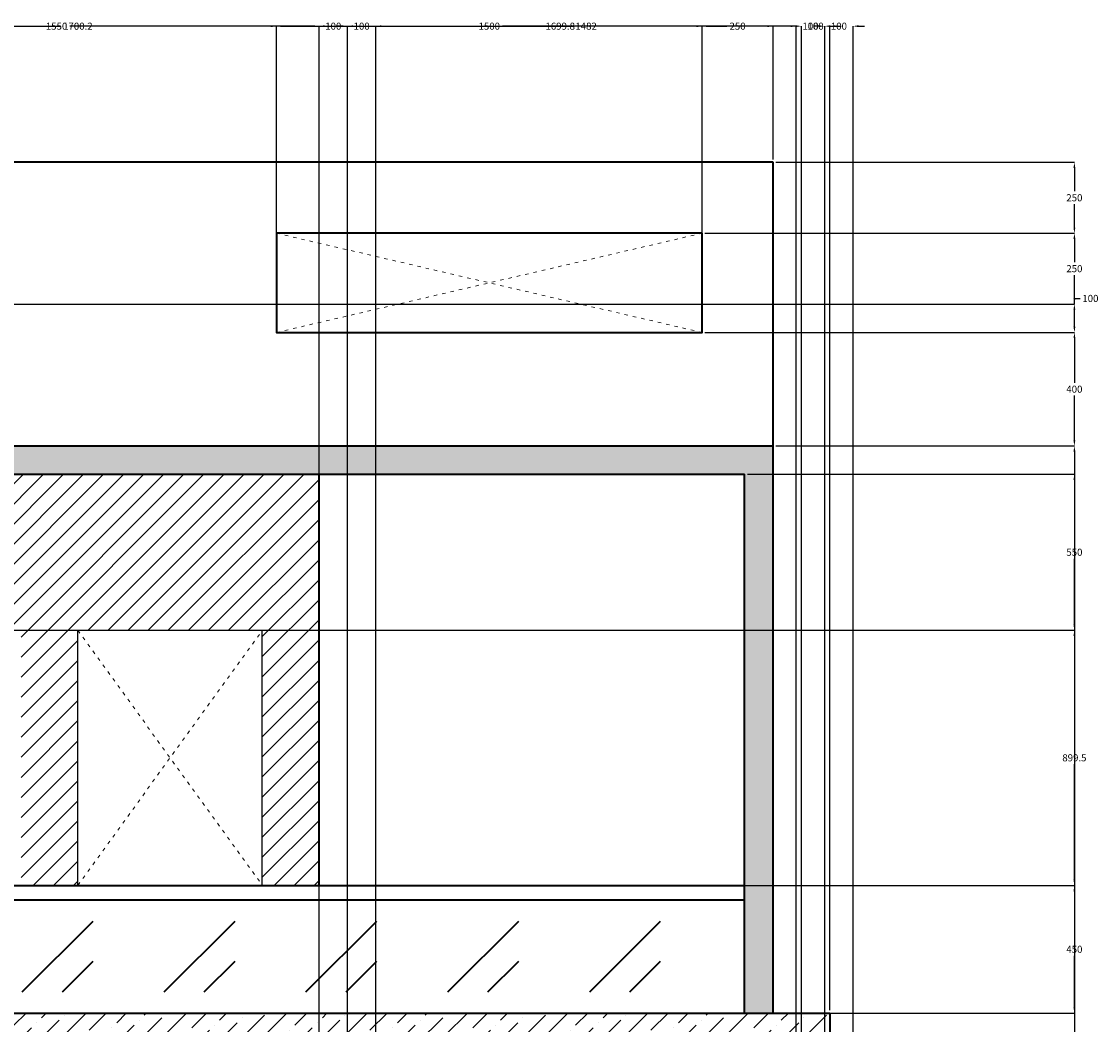
# Model space of a CAD drawing. Units: millimetres. Extents: x -692 to 9639, y -141 to 10345.
# Tile 19 of 19: x 5843 to 9639, y 6809 to 10345. Entities that reach past the tile are written whole.
import ezdxf

# ---------------------------------------------------------------- set-up
doc = ezdxf.new("R2010")
doc.units = ezdxf.units.MM
doc.header["$MEASUREMENT"] = 0
doc.linetypes.add('ACAD_ISO03W100', pattern=[30, 12, -18])
for name, color, linetype, lineweight in [('A-ANNO-DIMS', 2, 'Continuous', 18), ('A-DOOR', 3, 'Continuous', 25), ('A-DOOR-SWNG', 3, 'ACAD_ISO03W100', 18), ('A-ELEV', 7, 'Continuous', 35), ('A-ELEV-PATT', 8, 'Continuous', 13)]:
    doc.layers.add(name, color=color, linetype=linetype, lineweight=lineweight)
doc.styles.get("Standard").update_dxf_attribs({"font": 'arial.ttf'})
doc.dimstyles.get("Standard").update_dxf_attribs({"dimtxt": 25, "dimasz": 20, "dimexe": 0.18, "dimexo": 10, "dimgap": 10, "dimtad": 0, "dimtih": 1, "dimtoh": 1, "dimdec": 0, "dimzin": 0, "dimdsep": 46, "dimtxsty": 'Standard', "dimcen": 10, "dimadec": 0, "dimazin": 0, "dimtfac": 1, "dimtdec": 0, "dimtofl": 0, "dimtmove": 0, "dimatfit": 3, "dimfxl": 1, "dimtolj": 1, "dimtzin": 0, "dimarcsym": 0})

# ---------------------------------------------------------------- blocks, each defined once
blk = doc.blocks.new('*D7')
at = {"layer": 'A-ANNO-DIMS', "color": 0, "lineweight": -2, "transparency": 16777216}
for p, q in [((8481.5, 9848.8), (-649.1, 9848.8)), ((-648.9, 9828.8), (-648.9, 5124.9)), ((-648.9, 375.6), (-648.9, 5079.4)), ((2463.7, 355.6), (-649.1, 355.6))]:
    blk.add_line(p, q, dxfattribs=at)
at = {"layer": 'A-ANNO-DIMS', "color": 0, "lineweight": -3, "transparency": 16777216}
for points in [[(-652.2, 9828.8), (-645.6, 9828.8), (-648.9, 9848.8)], [(-652.2, 375.6), (-645.6, 375.6), (-648.9, 355.6)]]:
    blk.add_solid(points, dxfattribs=at)
at = {"layer": 'Defpoints', "color": 0, "lineweight": -3, "transparency": 16777216}
for p in [(-648.9, 9848.8), (8491.5, 9848.8), (2473.7, 355.6)]:
    blk.add_point(p, dxfattribs=at)
at = {"layer": 'A-ANNO-DIMS', "color": 0, "transparency": 16777216, "insert": (-648.9, 5102.2), "char_height": 25, "attachment_point": 5}
blk.add_mtext('\\A1;9493', dxfattribs=at)
blk = doc.blocks.new('*D9')
at = {"layer": 'A-ANNO-DIMS', "color": 0, "lineweight": -2, "transparency": 16777216}
for p, q in [((8501.5, 8848.8), (9553.9, 8848.8)), ((9553.7, 8828.8), (9553.7, 4874.9)), ((9553.7, 875.6), (9553.7, 4829.4)), ((9083.7, 855.6), (9553.9, 855.6))]:
    blk.add_line(p, q, dxfattribs=at)
at = {"layer": 'A-ANNO-DIMS', "color": 0, "lineweight": -3, "transparency": 16777216}
for points in [[(9550.4, 8828.8), (9557.1, 8828.8), (9553.7, 8848.8)], [(9550.4, 875.6), (9557.1, 875.6), (9553.7, 855.6)]]:
    blk.add_solid(points, dxfattribs=at)
at = {"layer": 'Defpoints', "color": 0, "lineweight": -3, "transparency": 16777216}
for p in [(8491.5, 8848.8), (9553.7, 8848.8), (9073.7, 855.6)]:
    blk.add_point(p, dxfattribs=at)
at = {"layer": 'A-ANNO-DIMS', "color": 0, "transparency": 16777216, "insert": (9553.7, 4852.2), "char_height": 25, "attachment_point": 5}
blk.add_mtext('\\A1;7993', dxfattribs=at)
blk = doc.blocks.new('*D10')
at = {"layer": 'A-ANNO-DIMS', "color": 0, "lineweight": -2, "transparency": 16777216}
for p, q in [((8251.5, 9248.8), (9553.9, 9248.8)), ((9553.7, 9228.8), (9553.7, 9071.5)), ((9553.7, 8868.8), (9553.7, 9026)), ((8501.5, 8848.8), (9553.9, 8848.8))]:
    blk.add_line(p, q, dxfattribs=at)
at = {"layer": 'A-ANNO-DIMS', "color": 0, "lineweight": -3, "transparency": 16777216}
for points in [[(9550.4, 9228.8), (9557.1, 9228.8), (9553.7, 9248.8)], [(9550.4, 8868.8), (9557.1, 8868.8), (9553.7, 8848.8)]]:
    blk.add_solid(points, dxfattribs=at)
at = {"layer": 'Defpoints', "color": 0, "lineweight": -3, "transparency": 16777216}
for p in [(8241.5, 9248.8), (9553.7, 9248.8), (8491.5, 8848.8)]:
    blk.add_point(p, dxfattribs=at)
at = {"layer": 'A-ANNO-DIMS', "color": 0, "transparency": 16777216, "insert": (9553.7, 9048.8), "char_height": 25, "attachment_point": 5}
blk.add_mtext('\\A1;400', dxfattribs=at)
blk = doc.blocks.new('*D11')
at = {"layer": 'A-ANNO-DIMS', "color": 0, "lineweight": -2, "transparency": 16777216}
for p, q in [((5201.5, 9348.8), (9553.9, 9348.8)), ((9553.7, 9348.8), (9553.7, 9368.8)), ((9553.7, 9368.8), (9573.7, 9368.8)), ((9553.7, 9268.8), (9553.7, 9328.8)), ((8251.5, 9248.8), (9553.9, 9248.8))]:
    blk.add_line(p, q, dxfattribs=at)
at = {"layer": 'A-ANNO-DIMS', "color": 0, "lineweight": -3, "transparency": 16777216}
for points in [[(9550.4, 9328.8), (9557.1, 9328.8), (9553.7, 9348.8)], [(9550.4, 9268.8), (9557.1, 9268.8), (9553.7, 9248.8)]]:
    blk.add_solid(points, dxfattribs=at)
at = {"layer": 'Defpoints', "color": 0, "lineweight": -3, "transparency": 16777216}
for p in [(5191.5, 9348.8), (9553.7, 9348.8), (8241.5, 9248.8)]:
    blk.add_point(p, dxfattribs=at)
at = {"layer": 'A-ANNO-DIMS', "color": 0, "transparency": 16777216, "insert": (9610.1, 9368.8), "char_height": 25, "attachment_point": 5}
blk.add_mtext('\\A1;100', dxfattribs=at)
blk = doc.blocks.new('*D12')
at = {"layer": 'A-ANNO-DIMS', "color": 0, "lineweight": -2, "transparency": 16777216}
for p, q in [((8251.5, 9598.8), (9553.9, 9598.8)), ((9553.7, 9578.8), (9553.7, 9496.5)), ((9553.7, 9368.8), (9553.7, 9451)), ((5201.5, 9348.8), (9553.9, 9348.8))]:
    blk.add_line(p, q, dxfattribs=at)
at = {"layer": 'A-ANNO-DIMS', "color": 0, "lineweight": -3, "transparency": 16777216}
for points in [[(9550.4, 9578.8), (9557.1, 9578.8), (9553.7, 9598.8)], [(9550.4, 9368.8), (9557.1, 9368.8), (9553.7, 9348.8)]]:
    blk.add_solid(points, dxfattribs=at)
at = {"layer": 'Defpoints', "color": 0, "lineweight": -3, "transparency": 16777216}
for p in [(8241.5, 9598.8), (9553.7, 9598.8), (5191.5, 9348.8)]:
    blk.add_point(p, dxfattribs=at)
at = {"layer": 'A-ANNO-DIMS', "color": 0, "transparency": 16777216, "insert": (9553.7, 9473.8), "char_height": 25, "attachment_point": 5}
blk.add_mtext('\\A1;250', dxfattribs=at)
blk = doc.blocks.new('*D13')
at = {"layer": 'A-ANNO-DIMS', "color": 0, "lineweight": -2, "transparency": 16777216}
for p, q in [((8501.5, 9848.8), (9553.9, 9848.8)), ((9553.7, 9828.8), (9553.7, 9746.5)), ((9553.7, 9618.8), (9553.7, 9701)), ((8251.5, 9598.8), (9553.9, 9598.8))]:
    blk.add_line(p, q, dxfattribs=at)
at = {"layer": 'A-ANNO-DIMS', "color": 0, "lineweight": -3, "transparency": 16777216}
for points in [[(9550.4, 9828.8), (9557.1, 9828.8), (9553.7, 9848.8)], [(9550.4, 9618.8), (9557.1, 9618.8), (9553.7, 9598.8)]]:
    blk.add_solid(points, dxfattribs=at)
at = {"layer": 'Defpoints', "color": 0, "lineweight": -3, "transparency": 16777216}
for p in [(8491.5, 9848.8), (9553.7, 9848.8), (8241.5, 9598.8)]:
    blk.add_point(p, dxfattribs=at)
at = {"layer": 'A-ANNO-DIMS', "color": 0, "transparency": 16777216, "insert": (9553.7, 9723.8), "char_height": 25, "attachment_point": 5}
blk.add_mtext('\\A1;250', dxfattribs=at)
blk = doc.blocks.new('*D15')
at = {"layer": 'A-ANNO-DIMS', "color": 0, "lineweight": -2, "transparency": 16777216}
for p, q in [((5191.5, 9358.8), (5191.5, 10329)), ((5211.5, 10328.8), (5920.4, 10328.8)), ((6721.5, 10328.8), (6012.7, 10328.8)), ((6741.5, 9258.8), (6741.5, 10329))]:
    blk.add_line(p, q, dxfattribs=at)
at = {"layer": 'A-ANNO-DIMS', "color": 0, "lineweight": -3, "transparency": 16777216}
for points in [[(5211.5, 10332.1), (5211.5, 10325.4), (5191.5, 10328.8)], [(6721.5, 10332.1), (6721.5, 10325.4), (6741.5, 10328.8)]]:
    blk.add_solid(points, dxfattribs=at)
at = {"layer": 'Defpoints', "color": 0, "lineweight": -3, "transparency": 16777216}
for p in [(6741.5, 10328.8), (5191.5, 9348.8), (6741.5, 9248.8)]:
    blk.add_point(p, dxfattribs=at)
at = {"layer": 'A-ANNO-DIMS', "color": 0, "transparency": 16777216, "insert": (5966.5, 10328.8), "char_height": 25, "attachment_point": 5}
blk.add_mtext('\\A1;1550', dxfattribs=at)
blk = doc.blocks.new('*D16')
at = {"layer": 'A-ANNO-DIMS', "color": 0, "lineweight": -2, "transparency": 16777216}
for p, q in [((6741.5, 9258.8), (6741.5, 10329)), ((6761.5, 10328.8), (7445.4, 10328.8)), ((8221.5, 10328.8), (7537.7, 10328.8)), ((8241.5, 9258.8), (8241.5, 10329))]:
    blk.add_line(p, q, dxfattribs=at)
at = {"layer": 'A-ANNO-DIMS', "color": 0, "lineweight": -3, "transparency": 16777216}
for points in [[(6761.5, 10332.1), (6761.5, 10325.4), (6741.5, 10328.8)], [(8221.5, 10332.1), (8221.5, 10325.4), (8241.5, 10328.8)]]:
    blk.add_solid(points, dxfattribs=at)
at = {"layer": 'Defpoints', "color": 0, "lineweight": -3, "transparency": 16777216}
for p in [(8241.5, 10328.8), (6741.5, 9248.8), (8241.5, 9248.8)]:
    blk.add_point(p, dxfattribs=at)
at = {"layer": 'A-ANNO-DIMS', "color": 0, "transparency": 16777216, "insert": (7491.5, 10328.8), "char_height": 25, "attachment_point": 5}
blk.add_mtext('\\A1;1500', dxfattribs=at)
blk = doc.blocks.new('*D17')
at = {"layer": 'A-ANNO-DIMS', "color": 0, "lineweight": -2, "transparency": 16777216}
for p, q in [((8241.5, 9608.8), (8241.5, 10329)), ((8261.5, 10328.8), (8328.8, 10328.8)), ((8471.5, 10328.8), (8404.3, 10328.8)), ((8491.5, 9858.8), (8491.5, 10329))]:
    blk.add_line(p, q, dxfattribs=at)
at = {"layer": 'A-ANNO-DIMS', "color": 0, "lineweight": -3, "transparency": 16777216}
for points in [[(8261.5, 10332.1), (8261.5, 10325.4), (8241.5, 10328.8)], [(8471.5, 10332.1), (8471.5, 10325.4), (8491.5, 10328.8)]]:
    blk.add_solid(points, dxfattribs=at)
at = {"layer": 'Defpoints', "color": 0, "lineweight": -3, "transparency": 16777216}
for p in [(8491.5, 10328.8), (8491.5, 9848.8), (8241.5, 9598.8)]:
    blk.add_point(p, dxfattribs=at)
at = {"layer": 'A-ANNO-DIMS', "color": 0, "transparency": 16777216, "insert": (8366.5, 10328.8), "char_height": 25, "attachment_point": 5}
blk.add_mtext('\\A1;250', dxfattribs=at)
blk = doc.blocks.new('*D32')
at = {"layer": 'A-ANNO-DIMS', "color": 0, "lineweight": -2, "transparency": 16777216}
for p, q in [((6871.7, 10328.8), (6851.7, 10328.8)), ((6891.7, 1865.6), (6891.7, 10329)), ((6991.7, 1765.6), (6991.7, 10329)), ((7011.7, 10328.8), (7031.7, 10328.8))]:
    blk.add_line(p, q, dxfattribs=at)
at = {"layer": 'A-ANNO-DIMS', "color": 0, "lineweight": -3, "transparency": 16777216}
for points in [[(6871.7, 10332.1), (6871.7, 10325.4), (6891.7, 10328.8)], [(7011.7, 10332.1), (7011.7, 10325.4), (6991.7, 10328.8)]]:
    blk.add_solid(points, dxfattribs=at)
at = {"layer": 'Defpoints', "color": 0, "lineweight": -3, "transparency": 16777216}
for p in [(6991.7, 10328.8), (6891.7, 1855.6), (6991.7, 1755.6)]:
    blk.add_point(p, dxfattribs=at)
at = {"layer": 'A-ANNO-DIMS', "color": 0, "transparency": 16777216, "insert": (6941.7, 10328.8), "char_height": 25, "attachment_point": 5}
blk.add_mtext('\\A1;100', dxfattribs=at)
blk = doc.blocks.new('*D33')
at = {"layer": 'A-ANNO-DIMS', "color": 0, "lineweight": -2, "transparency": 16777216}
for p, q in [((6971.7, 10328.8), (6951.7, 10328.8)), ((6991.7, 1765.6), (6991.7, 10329)), ((7091.7, 1665.6), (7091.7, 10329)), ((7111.7, 10328.8), (7131.7, 10328.8))]:
    blk.add_line(p, q, dxfattribs=at)
at = {"layer": 'A-ANNO-DIMS', "color": 0, "lineweight": -3, "transparency": 16777216}
for points in [[(6971.7, 10332.1), (6971.7, 10325.4), (6991.7, 10328.8)], [(7111.7, 10332.1), (7111.7, 10325.4), (7091.7, 10328.8)]]:
    blk.add_solid(points, dxfattribs=at)
at = {"layer": 'Defpoints', "color": 0, "lineweight": -3, "transparency": 16777216}
for p in [(7091.7, 10328.8), (6991.7, 1755.6), (7091.7, 1655.6)]:
    blk.add_point(p, dxfattribs=at)
at = {"layer": 'A-ANNO-DIMS', "color": 0, "transparency": 16777216, "insert": (7041.7, 10328.8), "char_height": 25, "attachment_point": 5}
blk.add_mtext('\\A1;100', dxfattribs=at)
blk = doc.blocks.new('*D34')
at = {"layer": 'A-ANNO-DIMS', "color": 0, "lineweight": -2, "transparency": 16777216}
for p, q in [((7091.7, 1665.6), (7091.7, 10329)), ((7111.7, 10328.8), (7786.7, 10328.8)), ((8553.7, 10328.8), (7878.8, 10328.8)), ((8573.7, 1665.6), (8573.7, 10329))]:
    blk.add_line(p, q, dxfattribs=at)
at = {"layer": 'A-ANNO-DIMS', "color": 0, "lineweight": -3, "transparency": 16777216}
for points in [[(7111.7, 10332.1), (7111.7, 10325.4), (7091.7, 10328.8)], [(8553.7, 10332.1), (8553.7, 10325.4), (8573.7, 10328.8)]]:
    blk.add_solid(points, dxfattribs=at)
at = {"layer": 'Defpoints', "color": 0, "lineweight": -3, "transparency": 16777216}
for p in [(8573.7, 10328.8), (7091.7, 1655.6), (8573.7, 1655.6)]:
    blk.add_point(p, dxfattribs=at)
at = {"layer": 'A-ANNO-DIMS', "color": 0, "transparency": 16777216, "insert": (7832.7, 10328.8), "char_height": 25, "attachment_point": 5}
blk.add_mtext('\\A1;1482', dxfattribs=at)
blk = doc.blocks.new('*D35')
at = {"layer": 'A-ANNO-DIMS', "color": 0, "lineweight": -2, "transparency": 16777216}
for p, q in [((8553.7, 10328.8), (8533.7, 10328.8)), ((8573.7, 1665.6), (8573.7, 10329)), ((8673.7, 1765.6), (8673.7, 10329)), ((8693.7, 10328.8), (8713.7, 10328.8))]:
    blk.add_line(p, q, dxfattribs=at)
at = {"layer": 'A-ANNO-DIMS', "color": 0, "lineweight": -3, "transparency": 16777216}
for points in [[(8553.7, 10332.1), (8553.7, 10325.4), (8573.7, 10328.8)], [(8693.7, 10332.1), (8693.7, 10325.4), (8673.7, 10328.8)]]:
    blk.add_solid(points, dxfattribs=at)
at = {"layer": 'Defpoints', "color": 0, "lineweight": -3, "transparency": 16777216}
for p in [(8673.7, 10328.8), (8673.7, 1755.6), (8573.7, 1655.6)]:
    blk.add_point(p, dxfattribs=at)
at = {"layer": 'A-ANNO-DIMS', "color": 0, "transparency": 16777216, "insert": (8623.7, 10328.8), "char_height": 25, "attachment_point": 5}
blk.add_mtext('\\A1;100', dxfattribs=at)
blk = doc.blocks.new('*D36')
at = {"layer": 'A-ANNO-DIMS', "color": 0, "lineweight": -2, "transparency": 16777216}
for p, q in [((8653.7, 10328.8), (8633.7, 10328.8)), ((8673.7, 1765.6), (8673.7, 10329)), ((8773.7, 1865.6), (8773.7, 10329)), ((8793.7, 10328.8), (8813.7, 10328.8))]:
    blk.add_line(p, q, dxfattribs=at)
at = {"layer": 'A-ANNO-DIMS', "color": 0, "lineweight": -3, "transparency": 16777216}
for points in [[(8653.7, 10332.1), (8653.7, 10325.4), (8673.7, 10328.8)], [(8793.7, 10332.1), (8793.7, 10325.4), (8773.7, 10328.8)]]:
    blk.add_solid(points, dxfattribs=at)
at = {"layer": 'Defpoints', "color": 0, "lineweight": -3, "transparency": 16777216}
for p in [(8773.7, 10328.8), (8773.7, 1855.6), (8673.7, 1755.6)]:
    blk.add_point(p, dxfattribs=at)
at = {"layer": 'A-ANNO-DIMS', "color": 0, "transparency": 16777216, "insert": (8723.7, 10328.8), "char_height": 25, "attachment_point": 5}
blk.add_mtext('\\A1;100', dxfattribs=at)
blk = doc.blocks.new('*D56')
at = {"layer": 'A-ANNO-DIMS', "color": 0, "lineweight": -2, "transparency": 16777216}
for p, q in [((5191.5, 6358.8), (5191.5, 10329)), ((5211.5, 10328.8), (5981.1, 10328.8)), ((6871.7, 10328.8), (6102.2, 10328.8)), ((6891.7, 6708.8), (6891.7, 10329))]:
    blk.add_line(p, q, dxfattribs=at)
at = {"layer": 'A-ANNO-DIMS', "color": 0, "lineweight": -3, "transparency": 16777216}
for points in [[(5211.5, 10332.1), (5211.5, 10325.4), (5191.5, 10328.8)], [(6871.7, 10332.1), (6871.7, 10325.4), (6891.7, 10328.8)]]:
    blk.add_solid(points, dxfattribs=at)
at = {"layer": 'Defpoints', "color": 0, "lineweight": -3, "transparency": 16777216}
for p in [(6891.7, 10328.8), (6891.7, 6698.8), (5191.5, 6348.8)]:
    blk.add_point(p, dxfattribs=at)
at = {"layer": 'A-ANNO-DIMS', "color": 0, "transparency": 16777216, "insert": (6041.6, 10328.8), "char_height": 25, "attachment_point": 5}
blk.add_mtext('\\A1;1700.2', dxfattribs=at)
blk = doc.blocks.new('*D57')
at = {"layer": 'A-ANNO-DIMS', "color": 0, "lineweight": -2, "transparency": 16777216}
for p, q in [((6891.7, 6708.8), (6891.7, 10329)), ((6911.7, 10328.8), (7680.9, 10328.8)), ((8571.5, 10328.8), (7802.4, 10328.8)), ((8591.5, 6708.8), (8591.5, 10329))]:
    blk.add_line(p, q, dxfattribs=at)
at = {"layer": 'A-ANNO-DIMS', "color": 0, "lineweight": -3, "transparency": 16777216}
for points in [[(6911.7, 10332.1), (6911.7, 10325.4), (6891.7, 10328.8)], [(8571.5, 10332.1), (8571.5, 10325.4), (8591.5, 10328.8)]]:
    blk.add_solid(points, dxfattribs=at)
at = {"layer": 'Defpoints', "color": 0, "lineweight": -3, "transparency": 16777216}
for p in [(8591.5, 10328.8), (6891.7, 6698.8), (8591.5, 6698.8)]:
    blk.add_point(p, dxfattribs=at)
at = {"layer": 'A-ANNO-DIMS', "color": 0, "transparency": 16777216, "insert": (7741.6, 10328.8), "char_height": 25, "attachment_point": 5}
blk.add_mtext('\\A1;1699.8', dxfattribs=at)
blk = doc.blocks.new('*D58')
at = {"layer": 'A-ANNO-DIMS', "color": 0, "lineweight": -2, "transparency": 16777216}
for p, q in [((8571.5, 10328.8), (8551.5, 10328.8)), ((8591.5, 6708.8), (8591.5, 10329)), ((8691.5, 6858.8), (8691.5, 10329)), ((8711.5, 10328.8), (8731.5, 10328.8))]:
    blk.add_line(p, q, dxfattribs=at)
at = {"layer": 'A-ANNO-DIMS', "color": 0, "lineweight": -3, "transparency": 16777216}
for points in [[(8571.5, 10332.1), (8571.5, 10325.4), (8591.5, 10328.8)], [(8711.5, 10332.1), (8711.5, 10325.4), (8691.5, 10328.8)]]:
    blk.add_solid(points, dxfattribs=at)
at = {"layer": 'Defpoints', "color": 0, "lineweight": -3, "transparency": 16777216}
for p in [(8691.5, 10328.8), (8691.5, 6848.8), (8591.5, 6698.8)]:
    blk.add_point(p, dxfattribs=at)
at = {"layer": 'A-ANNO-DIMS', "color": 0, "transparency": 16777216, "insert": (8641.5, 10328.8), "char_height": 25, "attachment_point": 5}
blk.add_mtext('\\A1;100', dxfattribs=at)
blk = doc.blocks.new('*D76')
at = {"layer": 'A-ANNO-DIMS', "color": 0, "lineweight": -2, "transparency": 16777216}
for p, q in [((5101.5, 7298.8), (9553.9, 7298.8)), ((9553.7, 7278.8), (9553.7, 7096.5)), ((9553.7, 6868.8), (9553.7, 7051)), ((5101.5, 6848.8), (9553.9, 6848.8))]:
    blk.add_line(p, q, dxfattribs=at)
at = {"layer": 'A-ANNO-DIMS', "color": 0, "lineweight": -3, "transparency": 16777216}
for points in [[(9550.4, 7278.8), (9557.1, 7278.8), (9553.7, 7298.8)], [(9550.4, 6868.8), (9557.1, 6868.8), (9553.7, 6848.8)]]:
    blk.add_solid(points, dxfattribs=at)
at = {"layer": 'Defpoints', "color": 0, "lineweight": -3, "transparency": 16777216}
for p in [(5091.5, 7298.8), (9553.7, 7298.8), (5091.5, 6848.8)]:
    blk.add_point(p, dxfattribs=at)
at = {"layer": 'A-ANNO-DIMS', "color": 0, "transparency": 16777216, "insert": (9553.7, 7073.8), "char_height": 25, "attachment_point": 5}
blk.add_mtext('\\A1;450', dxfattribs=at)
blk = doc.blocks.new('*D77')
at = {"layer": 'A-ANNO-DIMS', "color": 0, "lineweight": -2, "transparency": 16777216}
for p, q in [((5201.5, 8198.8), (9553.9, 8198.8)), ((9553.7, 8178.8), (9553.7, 7771.8)), ((9553.7, 7319.3), (9553.7, 7726.3)), ((5201.5, 7299.3), (9553.9, 7299.3))]:
    blk.add_line(p, q, dxfattribs=at)
at = {"layer": 'A-ANNO-DIMS', "color": 0, "lineweight": -3, "transparency": 16777216}
for points in [[(9550.4, 8178.8), (9557.1, 8178.8), (9553.7, 8198.8)], [(9550.4, 7319.3), (9557.1, 7319.3), (9553.7, 7299.3)]]:
    blk.add_solid(points, dxfattribs=at)
at = {"layer": 'Defpoints', "color": 0, "lineweight": -3, "transparency": 16777216}
for p in [(5191.5, 8198.8), (9553.7, 8198.8), (5191.5, 7299.3)]:
    blk.add_point(p, dxfattribs=at)
at = {"layer": 'A-ANNO-DIMS', "color": 0, "transparency": 16777216, "insert": (9553.7, 7749), "char_height": 25, "attachment_point": 5}
blk.add_mtext('\\A1;899.5', dxfattribs=at)
blk = doc.blocks.new('*D78')
at = {"layer": 'A-ANNO-DIMS', "color": 0, "lineweight": -2, "transparency": 16777216}
for p, q in [((8401.5, 8748.8), (9553.9, 8748.8)), ((9553.7, 8728.8), (9553.7, 8496.5)), ((9553.7, 8218.8), (9553.7, 8451)), ((5201.5, 8198.8), (9553.9, 8198.8))]:
    blk.add_line(p, q, dxfattribs=at)
at = {"layer": 'A-ANNO-DIMS', "color": 0, "lineweight": -3, "transparency": 16777216}
for points in [[(9550.4, 8728.8), (9557.1, 8728.8), (9553.7, 8748.8)], [(9550.4, 8218.8), (9557.1, 8218.8), (9553.7, 8198.8)]]:
    blk.add_solid(points, dxfattribs=at)
at = {"layer": 'Defpoints', "color": 0, "lineweight": -3, "transparency": 16777216}
for p in [(8391.5, 8748.8), (9553.7, 8748.8), (5191.5, 8198.8)]:
    blk.add_point(p, dxfattribs=at)
at = {"layer": 'A-ANNO-DIMS', "color": 0, "transparency": 16777216, "insert": (9553.7, 8473.8), "char_height": 25, "attachment_point": 5}
blk.add_mtext('\\A1;550', dxfattribs=at)

msp = doc.modelspace()

# ---------------------------------------------------------------- hatches: boundary and pattern name
at = {"layer": 'A-ELEV-PATT'}
h = msp.add_hatch(dxfattribs=at)
h.set_pattern_fill('CROSS', color=256, scale=150)
h.paths.add_polyline_path([(8491.547, 8848.772), (3791.547, 8848.772), (3791.547, 8748.772), (8391.547, 8748.772), (8391.547, 6848.772), (8491.547, 6848.772)])
h = msp.add_hatch(dxfattribs=at)
h.set_pattern_fill('ANSI31', color=256, scale=400)
h.paths.add_polyline_path([(6891.746, 6698.772), (5191.547, 6698.772), (5191.547, 6348.772), (5841.547, 6348.772), (5841.547, 5448.772), (6041.547, 5448.772), (6041.547, 6348.772), (6691.547, 6348.772), (6691.547, 5448.772), (6891.746, 5448.772)])
h.paths.add_polyline_path([(5191.547, 6698.772), (3941.547, 6698.772), (3941.547, 5448.772), (4006.259, 5448.772), (4006.259, 6423.772), (5081.259, 6423.772), (5081.259, 5448.772), (5191.547, 5448.772), (5191.547, 6348.772)])
h.paths.add_polyline_path([(6891.746, 4848.772), (5191.547, 4848.772), (5191.547, 4497.772), (5841.746, 4497.772), (5841.746, 3598.27), (6041.746, 3598.27), (6041.746, 4497.772), (6691.746, 4497.772), (6691.746, 3598.27), (6891.746, 3598.27)])
h.paths.add_polyline_path([(6891.746, 8748.772), (5191.547, 8748.772), (5191.547, 8198.772), (5841.547, 8198.772), (5841.547, 7298.772), (6041.547, 7298.772), (6041.547, 8198.772), (6691.547, 8198.772), (6691.547, 7298.772), (6891.746, 7298.772)])
h = msp.add_hatch(dxfattribs=at)
h.set_pattern_fill('ANSI36', color=256, scale=400)
h.paths.add_polyline_path([(8691.547, 6848.772), (3791.547, 6848.772), (3791.547, 4848.772), (8691.547, 4848.772), (8691.547, 4998.772), (3941.547, 4998.772), (3941.547, 6698.772), (8691.547, 6698.772)])

# ---------------------------------------------------------------- linework, layer by layer
at = {"layer": 'A-DOOR'}
for p, q in [((6041.547, 7298.772), (6041.547, 8198.772)), ((6041.547, 8198.772), (6691.547, 8198.772)), ((6691.547, 7298.772), (6691.547, 8198.772))]:
    msp.add_line(p, q, dxfattribs=at)
at = {"layer": 'A-DOOR-SWNG'}
for p, q in [((6741.547, 9248.772), (8241.547, 9598.772)), ((6741.547, 9598.772), (8241.547, 9248.772)), ((6041.547, 7299.27), (6691.746, 8198.772)), ((6041.547, 8198.772), (6691.746, 7299.27))]:
    msp.add_line(p, q, dxfattribs=at)
at = {"layer": 'A-ELEV'}
for p, q in [((8491.547, 9848.772), (4991.547, 9848.772)), ((8491.547, 8848.772), (8491.547, 9848.772)), ((3791.547, 8848.772), (8491.547, 8848.772)), ((8491.547, 6848.772), (8491.547, 8848.772)), ((3791.547, 8748.772), (8391.547, 8748.772)), ((6891.746, 7298.772), (6891.746, 8748.772)), ((8391.547, 6848.772), (8391.547, 8748.772)), ((5191.547, 7298.772), (8391.547, 7298.772)), ((5091.547, 7248.772), (8391.547, 7248.772)), ((6094.403, 7172.266), (5844.403, 6922.266)), ((6594.403, 7172.266), (6344.403, 6922.266)), ((7094.403, 7172.266), (6844.403, 6922.266)), ((7594.403, 7172.266), (7344.403, 6922.266)), ((8094.403, 7172.266), (7844.403, 6922.266)), ((6094.403, 7030.844), (5985.824, 6922.266)), ((6594.403, 7030.844), (6485.824, 6922.266)), ((7094.403, 7030.844), (6985.824, 6922.266)), ((7594.403, 7030.844), (7485.824, 6922.266)), ((8094.403, 7030.844), (7985.824, 6922.266)), ((3791.547, 6848.772), (8691.547, 6848.772)), ((8691.547, 6848.772), (8691.547, 6698.772))]:
    msp.add_line(p, q, dxfattribs=at)
msp.add_lwpolyline([(8241.547, 9598.772), (6741.547, 9598.772), (6741.547, 9248.772), (8241.547, 9248.772)], close=True, dxfattribs=at)

# ---------------------------------------------------------------- dimensions: what is measured, and where the dimension line sits
at = {"layer": 'A-ANNO-DIMS'}
for base, p1, p2, override, picture, middle in [((6741.547, 10328.772), (5191.547, 9348.772), (6741.547, 9248.772), {"dimdec": 0, "dimlfac": 1, "dimrnd": 0, "dimzin": 0, "dimdsep": 46, "dimlunit": 2}, '*D15', (5966.547, 10328.772)), ((6891.746, 10328.772), (5191.547, 6348.772), (6891.746, 6698.772), {"dimdec": 1, "dimlfac": 1, "dimrnd": 0, "dimzin": 0, "dimdsep": 46, "dimlunit": 2}, '*D56', (6041.646, 10328.772)), ((8241.547, 10328.772), (6741.547, 9248.772), (8241.547, 9248.772), {"dimdec": 0, "dimlfac": 1, "dimrnd": 0, "dimzin": 0, "dimdsep": 46, "dimlunit": 2}, '*D16', (7491.547, 10328.772)), ((6991.746, 10328.772), (6891.746, 1855.575), (6991.746, 1755.575), {"dimdec": 0, "dimlfac": 1, "dimrnd": 0, "dimzin": 0, "dimdsep": 46, "dimlunit": 2}, '*D32', (6941.746, 10328.772)), ((8591.547, 10328.772), (6891.746, 6698.772), (8591.547, 6698.772), {"dimdec": 1, "dimlfac": 1, "dimrnd": 0, "dimzin": 0, "dimdsep": 46, "dimlunit": 2}, '*D57', (7741.646, 10328.772)), ((7091.746, 10328.772), (6991.746, 1755.575), (7091.746, 1655.575), {"dimdec": 0, "dimlfac": 1, "dimrnd": 0, "dimzin": 0, "dimdsep": 46, "dimlunit": 2}, '*D33', (7041.746, 10328.772)), ((8573.746, 10328.772), (7091.746, 1655.575), (8573.746, 1655.575), {"dimdec": 0, "dimlfac": 1, "dimrnd": 0, "dimzin": 0, "dimdsep": 46, "dimlunit": 2}, '*D34', (7832.746, 10328.772)), ((8491.547, 10328.772), (8241.547, 9598.772), (8491.547, 9848.772), {"dimdec": 0, "dimlfac": 1, "dimrnd": 0, "dimzin": 0, "dimdsep": 46, "dimlunit": 2}, '*D17', (8366.547, 10328.772)), ((8673.746, 10328.772), (8573.746, 1655.575), (8673.746, 1755.575), {"dimdec": 0, "dimlfac": 1, "dimrnd": 0, "dimzin": 0, "dimdsep": 46, "dimlunit": 2}, '*D35', (8623.746, 10328.772)), ((8691.547, 10328.772), (8591.547, 6698.772), (8691.547, 6848.772), {"dimdec": 0, "dimlfac": 1, "dimrnd": 0, "dimzin": 0, "dimdsep": 46, "dimlunit": 2}, '*D58', (8641.547, 10328.772)), ((8773.746, 10328.772), (8673.746, 1755.575), (8773.746, 1855.575), {"dimdec": 0, "dimlfac": 1, "dimrnd": 0, "dimzin": 0, "dimdsep": 46, "dimlunit": 2}, '*D36', (8723.746, 10328.772))]:
    dim = msp.add_linear_dim(base=base, p1=p1, p2=p2, dimstyle='Standard', override=override, dxfattribs=at)
    dim.commit()
    dim.dimension.update_dxf_attribs({"geometry": picture, "text_midpoint": middle})
for base, p1, p2, override, picture, middle in [((-648.912, 9848.772), (2473.746, 355.575), (8491.547, 9848.772), {"dimdec": 0, "dimlfac": 1, "dimrnd": 0, "dimzin": 0, "dimdsep": 46, "dimlunit": 2}, '*D7', (-648.912, 5102.173)), ((9553.746, 9848.772), (8241.547, 9598.772), (8491.547, 9848.772), {"dimdec": 0, "dimlfac": 1, "dimrnd": 0, "dimzin": 0, "dimdsep": 46, "dimlunit": 2}, '*D13', (9553.746, 9723.772)), ((9553.746, 9598.772), (5191.547, 9348.772), (8241.547, 9598.772), {"dimdec": 0, "dimlfac": 1, "dimrnd": 0, "dimzin": 0, "dimdsep": 46, "dimlunit": 2}, '*D12', (9553.746, 9473.772)), ((9553.746, 9348.772), (8241.547, 9248.772), (5191.547, 9348.772), {"dimdec": 0, "dimlfac": 1, "dimrnd": 0, "dimzin": 0, "dimdsep": 46, "dimlunit": 2}, '*D11', (9610.144, 9368.772)), ((9553.746, 9248.772), (8491.547, 8848.772), (8241.547, 9248.772), {"dimdec": 0, "dimlfac": 1, "dimrnd": 0, "dimzin": 0, "dimdsep": 46, "dimlunit": 2}, '*D10', (9553.746, 9048.772)), ((9553.746, 8848.772), (9073.746, 855.575), (8491.547, 8848.772), {"dimdec": 0, "dimlfac": 1, "dimrnd": 0, "dimzin": 0, "dimdsep": 46, "dimlunit": 2}, '*D9', (9553.746, 4852.173)), ((9553.746, 8748.772), (5191.547, 8198.772), (8391.547, 8748.772), {"dimdec": 0, "dimlfac": 1, "dimrnd": 0, "dimzin": 0, "dimdsep": 46, "dimlunit": 2}, '*D78', (9553.746, 8473.772)), ((9553.746, 8198.772), (5191.547, 7299.27), (5191.547, 8198.772), {"dimdec": 1, "dimlfac": 1, "dimrnd": 0, "dimzin": 0, "dimdsep": 46, "dimlunit": 2}, '*D77', (9553.746, 7749.021)), ((9553.746, 7298.772), (5091.547, 6848.772), (5091.547, 7298.772), {"dimdec": 0, "dimlfac": 1, "dimrnd": 0, "dimzin": 0, "dimdsep": 46, "dimlunit": 2}, '*D76', (9553.746, 7073.772))]:
    dim = msp.add_linear_dim(base=base, p1=p1, p2=p2, angle=90, dimstyle='Standard', override=override, dxfattribs=at)
    dim.commit()
    dim.dimension.update_dxf_attribs({"geometry": picture, "text_midpoint": middle})

doc.saveas('drawing.dxf')
